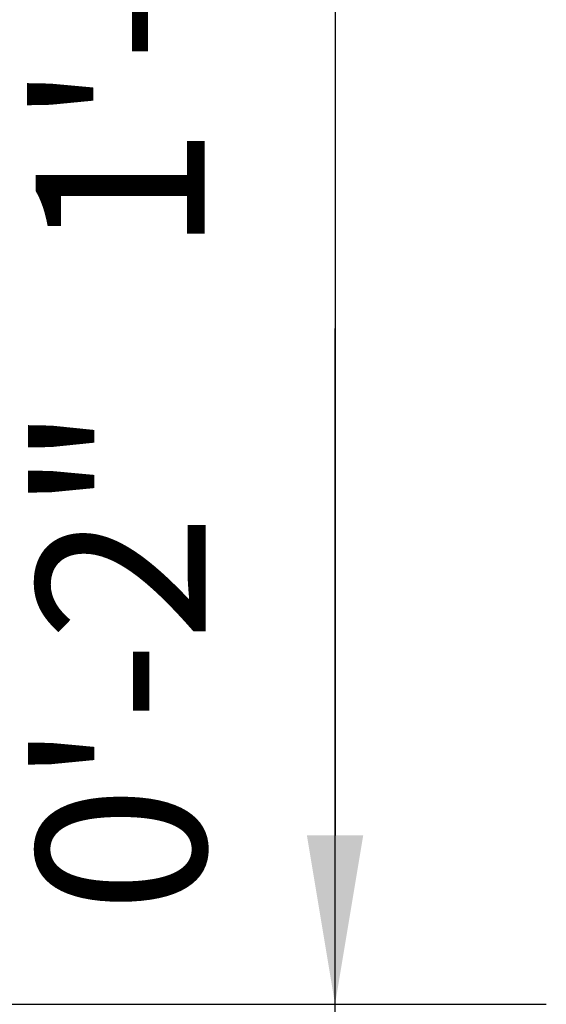
# Model space of a CAD drawing. Units: millimetres. Extents: x 7894 to 8038, y 6851 to 6951.
# Tile 41 of 49: x 7972.111 to 7975.227, y 6922.628 to 6928.457. Entities that reach past the tile are written whole.
import ezdxf

# ---------------------------------------------------------------- set-up
doc = ezdxf.new("R2010")
doc.units = ezdxf.units.MM
doc.layers.add('A-ANNO-DIMS', color=2, linetype='Continuous', lineweight=18)
doc.styles.get("Standard").update_dxf_attribs({"font": 'arial.ttf'})
doc.dimstyles.new('ISO-25', dxfattribs={"dimtxt": 1, "dimasz": 1, "dimexe": 1.25, "dimexo": 0.625, "dimtad": 1, "dimdec": 0, "dimlunit": 4, "dimtxsty": 'Standard', "dimcen": 2.5, "dimclrt": 1, "dimadec": 0, "dimazin": 0, "dimtfac": 1, "dimtdec": 0, "dimtmove": 0, "dimatfit": 3, "dimfxl": 1, "dimarcsym": 0})

# ---------------------------------------------------------------- blocks, each defined once
blk = doc.blocks.new('*D28')
at = {"layer": 'A-ANNO-DIMS', "color": 0, "lineweight": -2, "transparency": 16777216}
for p, q in [((7960.8854, 6936.8804), (7975.2272, 6936.8804)), ((7973.9772, 6935.8804), (7973.9772, 6923.6283)), ((7971.8421, 6922.6283), (7975.2272, 6922.6283))]:
    blk.add_line(p, q, dxfattribs=at)
at = {"layer": 'A-ANNO-DIMS', "color": 0, "transparency": 16777216}
for points in [[(7973.8105, 6935.8804), (7974.1439, 6935.8804), (7973.9772, 6936.8804)], [(7973.8105, 6923.6283), (7974.1439, 6923.6283), (7973.9772, 6922.6283)]]:
    blk.add_solid(points, dxfattribs=at)
at = {"layer": 'Defpoints', "color": 0, "transparency": 16777216}
for p in [(7960.2604, 6936.8804), (7971.2171, 6922.6283), (7973.9772, 6922.6283)]:
    blk.add_point(p, dxfattribs=at)
at = {"layer": 'A-ANNO-DIMS', "color": 1, "transparency": 16777216, "insert": (7972.8351, 6929.7543), "char_height": 1, "attachment_point": 5, "rotation": 90}
blk.add_mtext('1\'-2 1/2"', dxfattribs=at)
blk = doc.blocks.new('*D31')
at = {"layer": 'A-ANNO-DIMS', "color": 0, "lineweight": -2, "transparency": 16777216}
for p, q in [((7973.9772, 6921.7198), (7973.9772, 6926.628)), ((7949.8107, 6920.7198), (7975.2272, 6920.7198)), ((7973.9772, 6918.7198), (7973.9772, 6920.7198)), ((7950.9654, 6918.7198), (7975.2272, 6918.7198)), ((7973.9772, 6917.7198), (7973.9772, 6916.7198))]:
    blk.add_line(p, q, dxfattribs=at)
at = {"layer": 'A-ANNO-DIMS', "color": 0, "transparency": 16777216}
for points in [[(7973.8105, 6921.7198), (7974.1439, 6921.7198), (7973.9772, 6920.7198)], [(7973.8105, 6917.7198), (7974.1439, 6917.7198), (7973.9772, 6918.7198)]]:
    blk.add_solid(points, dxfattribs=at)
at = {"layer": 'Defpoints', "color": 0, "transparency": 16777216}
for p in [(7949.1857, 6920.7198), (7973.9772, 6920.7198), (7950.3404, 6918.7198)]:
    blk.add_point(p, dxfattribs=at)
at = {"layer": 'A-ANNO-DIMS', "color": 1, "transparency": 16777216, "insert": (7972.8416, 6924.6739), "char_height": 1, "attachment_point": 5, "rotation": 90}
blk.add_mtext('0\'-2"', dxfattribs=at)

msp = doc.modelspace()

# ---------------------------------------------------------------- dimensions: what is measured, and where the dimension line sits
at = {"layer": 'A-ANNO-DIMS'}
for base, p1, p2, picture, middle in [((7973.9772, 6922.6283), (7960.2604, 6936.8804), (7971.2171, 6922.6283), '*D28', (7972.8351, 6929.7543)), ((7973.9772, 6920.7198), (7950.3404, 6918.7198), (7949.1857, 6920.7198), '*D31', (7972.8416, 6924.6739))]:
    dim = msp.add_linear_dim(base=base, p1=p1, p2=p2, angle=90, dimstyle='ISO-25', override={"dimdec": 1, "dimlfac": 1, "dimrnd": 0, "dimzin": 1, "dimdsep": 46, "dimlunit": 4, "dimfrac": 2}, dxfattribs=at)
    dim.commit()
    dim.dimension.update_dxf_attribs({"geometry": picture, "text_midpoint": middle})

doc.saveas('drawing.dxf')
